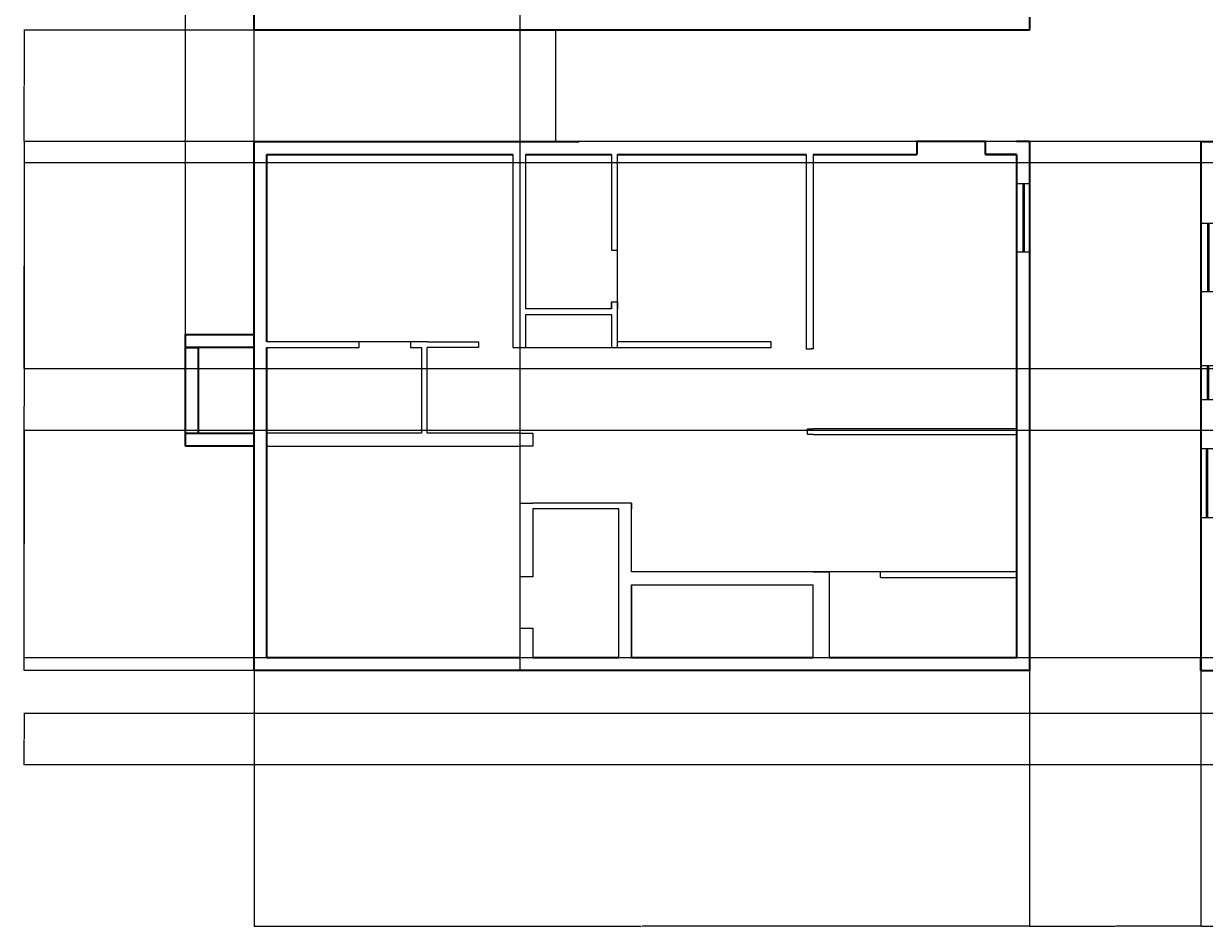
# Model space of a CAD drawing. Units: inches. Extents: x 2029 to 8798, y 1998 to 6373.
# Tile 1 of 11: x 2029 to 2855, y 4031 to 4662. Entities that reach past the tile are written whole.
import ezdxf

# ---------------------------------------------------------------- set-up
doc = ezdxf.new("R2010")
doc.units = ezdxf.units.IN
for name, color, linetype, lineweight in [('A-ANNO-DIMS', 2, 'Continuous', 18), ('A-GLAZ', 4, 'Continuous', 18), ('A-WALL-CIRC', 7, 'Continuous', 25), ('A-WALL-EXTR', 7, 'Continuous', 35), ('A-WALL-INTR', 7, 'Continuous', 25)]:
    doc.layers.add(name, color=color, linetype=linetype, lineweight=lineweight)
doc.styles.get("Standard").update_dxf_attribs({"font": 'arial.ttf'})
doc.dimstyles.get("Standard").update_dxf_attribs({"dimtxt": 0.18, "dimasz": 0.18, "dimexe": 0.18, "dimexo": 0.0625, "dimgap": 0.09, "dimtad": 0, "dimtih": 1, "dimtoh": 1, "dimdec": 4, "dimzin": 0, "dimdsep": 46, "dimtxsty": 'Standard', "dimcen": 0.09, "dimadec": 0, "dimazin": 0, "dimtfac": 1, "dimtdec": 4, "dimtofl": 0, "dimtmove": 0, "dimatfit": 3, "dimfxl": 1, "dimtolj": 1, "dimtzin": 0, "dimarcsym": 0})

# ---------------------------------------------------------------- blocks, each defined once
blk = doc.blocks.new('WIN-48')
for p, q in [((0, 48), (9, 48)), ((4.5, 48), (4.5, 0)), ((5.5, 48), (5.5, 0)), ((9, 0), (0, 0))]:
    blk.add_line(p, q)
blk = doc.blocks.new('WIN-24')
for p, q in [((0, 0), (0, 9)), ((24, 9), (24, 0)), ((0, 4.5), (24, 4.5)), ((0, 3.5), (24, 3.5))]:
    blk.add_line(p, q)
blk = doc.blocks.new('WALL-BAY-78X48')
for p, q in [((0, 69), (0, 78)), ((0, 78), (48, 78)), ((48, 69), (0, 69)), ((0, 9), (0, 69)), ((0, 69), (9, 69)), ((9, 69), (9, 9)), ((0, 0), (0, 9)), ((0, 9), (48, 9)), ((48, 0), (0, 0))]:
    blk.add_line(p, q)
blk = doc.blocks.new('*D37')
at = {"layer": 'A-ANNO-DIMS', "color": 0, "lineweight": -2, "transparency": 16777216}
for p, q in [((2190.54, 4209.93), (2190.54, 4031.06)), ((2732.54, 4209.93), (2732.54, 4031.06)), ((2190.72, 4031.24), (2461.25, 4031.24)), ((2732.36, 4031.24), (2461.83, 4031.24))]:
    blk.add_line(p, q, dxfattribs=at)
at = {"layer": 'A-ANNO-DIMS', "color": 0, "transparency": 16777216}
for points in [[(2190.72, 4031.27), (2190.72, 4031.21), (2190.54, 4031.24)], [(2732.36, 4031.27), (2732.36, 4031.21), (2732.54, 4031.24)]]:
    blk.add_solid(points, dxfattribs=at)
at = {"layer": 'Defpoints', "color": 0, "transparency": 16777216}
for p in [(2190.54, 4209.99), (2732.54, 4209.99), (2732.54, 4031.24)]:
    blk.add_point(p, dxfattribs=at)
at = {"layer": 'A-ANNO-DIMS', "color": 0, "transparency": 16777216, "insert": (2461.54, 4031.24), "char_height": 0.18, "attachment_point": 5}
blk.add_mtext('\\A1;542', dxfattribs=at)
blk = doc.blocks.new('*D38')
at = {"layer": 'A-ANNO-DIMS', "color": 0, "lineweight": -2, "transparency": 16777216}
for p, q in [((2732.54, 4209.93), (2732.54, 4031.06)), ((2852.54, 4209.93), (2852.54, 4031.06)), ((2732.72, 4031.24), (2792.26, 4031.24)), ((2852.36, 4031.24), (2792.82, 4031.24))]:
    blk.add_line(p, q, dxfattribs=at)
at = {"layer": 'A-ANNO-DIMS', "color": 0, "transparency": 16777216}
for points in [[(2732.72, 4031.27), (2732.72, 4031.21), (2732.54, 4031.24)], [(2852.36, 4031.27), (2852.36, 4031.21), (2852.54, 4031.24)]]:
    blk.add_solid(points, dxfattribs=at)
at = {"layer": 'Defpoints', "color": 0, "transparency": 16777216}
for p in [(2732.54, 4209.99), (2852.54, 4209.99), (2852.54, 4031.24)]:
    blk.add_point(p, dxfattribs=at)
at = {"layer": 'A-ANNO-DIMS', "color": 0, "transparency": 16777216, "insert": (2792.54, 4031.24), "char_height": 0.18, "attachment_point": 5}
blk.add_mtext('\\A1;120', dxfattribs=at)
blk = doc.blocks.new('*D39')
at = {"layer": 'A-ANNO-DIMS', "color": 0, "lineweight": -2, "transparency": 16777216}
for p, q in [((2852.54, 4209.93), (2852.54, 4031.06)), ((3252.54, 4209.93), (3252.54, 4031.06)), ((2852.72, 4031.24), (3052.25, 4031.24)), ((3252.36, 4031.24), (3052.83, 4031.24))]:
    blk.add_line(p, q, dxfattribs=at)
at = {"layer": 'A-ANNO-DIMS', "color": 0, "transparency": 16777216}
for points in [[(2852.72, 4031.27), (2852.72, 4031.21), (2852.54, 4031.24)], [(3252.36, 4031.27), (3252.36, 4031.21), (3252.54, 4031.24)]]:
    blk.add_solid(points, dxfattribs=at)
at = {"layer": 'Defpoints', "color": 0, "transparency": 16777216}
for p in [(2852.54, 4209.99), (3252.54, 4209.99), (3252.54, 4031.24)]:
    blk.add_point(p, dxfattribs=at)
at = {"layer": 'A-ANNO-DIMS', "color": 0, "transparency": 16777216, "insert": (3052.54, 4031.24), "char_height": 0.18, "attachment_point": 5}
blk.add_mtext('\\A1;400', dxfattribs=at)
blk = doc.blocks.new('*D43')
at = {"layer": 'A-ANNO-DIMS', "color": 0, "lineweight": -2, "transparency": 16777216}
for p, q in [((2190.48, 4579.99), (2029.61, 4579.99)), ((2029.79, 4579.81), (2029.79, 4395.17)), ((2029.79, 4210.17), (2029.79, 4394.81)), ((2190.48, 4209.99), (2029.61, 4209.99))]:
    blk.add_line(p, q, dxfattribs=at)
at = {"layer": 'A-ANNO-DIMS', "color": 0, "transparency": 16777216}
for points in [[(2029.76, 4579.81), (2029.82, 4579.81), (2029.79, 4579.99)], [(2029.76, 4210.17), (2029.82, 4210.17), (2029.79, 4209.99)]]:
    blk.add_solid(points, dxfattribs=at)
at = {"layer": 'Defpoints', "color": 0, "transparency": 16777216}
for p in [(2029.79, 4579.99), (2190.54, 4579.99), (2190.54, 4209.99)]:
    blk.add_point(p, dxfattribs=at)
at = {"layer": 'A-ANNO-DIMS', "color": 0, "transparency": 16777216, "insert": (2029.79, 4394.99), "char_height": 0.18, "attachment_point": 5}
blk.add_mtext('\\A1;370', dxfattribs=at)
blk = doc.blocks.new('*D44')
at = {"layer": 'A-ANNO-DIMS', "color": 0, "lineweight": -2, "transparency": 16777216}
for p, q in [((2190.48, 4657.96), (2029.61, 4657.96)), ((2029.79, 4657.78), (2029.79, 4619.16)), ((2029.79, 4580.17), (2029.79, 4618.79)), ((2190.48, 4579.99), (2029.61, 4579.99))]:
    blk.add_line(p, q, dxfattribs=at)
at = {"layer": 'A-ANNO-DIMS', "color": 0, "transparency": 16777216}
for points in [[(2029.76, 4657.78), (2029.82, 4657.78), (2029.79, 4657.96)], [(2029.76, 4580.17), (2029.82, 4580.17), (2029.79, 4579.99)]]:
    blk.add_solid(points, dxfattribs=at)
at = {"layer": 'Defpoints', "color": 0, "transparency": 16777216}
for p in [(2029.79, 4657.96), (2190.54, 4657.96), (2190.54, 4579.99)]:
    blk.add_point(p, dxfattribs=at)
at = {"layer": 'A-ANNO-DIMS', "color": 0, "transparency": 16777216, "insert": (2029.79, 4618.97), "char_height": 0.18, "attachment_point": 5}
blk.add_mtext('\\A1;77.97', dxfattribs=at)
blk = doc.blocks.new('*D49')
at = {"layer": 'A-ANNO-DIMS', "color": 0, "lineweight": -2, "transparency": 16777216}
for p, q in [((2190.54, 4210.05), (2190.54, 6372.54)), ((2190.72, 6372.36), (2283.26, 6372.36)), ((2376.36, 6372.36), (2283.82, 6372.36)), ((2376.54, 4210.05), (2376.54, 6372.54))]:
    blk.add_line(p, q, dxfattribs=at)
at = {"layer": 'A-ANNO-DIMS', "color": 0, "transparency": 16777216}
for points in [[(2190.72, 6372.39), (2190.72, 6372.33), (2190.54, 6372.36)], [(2376.36, 6372.39), (2376.36, 6372.33), (2376.54, 6372.36)]]:
    blk.add_solid(points, dxfattribs=at)
at = {"layer": 'Defpoints', "color": 0, "transparency": 16777216}
for p in [(2376.54, 6372.36), (2190.54, 4209.99), (2376.54, 4209.99)]:
    blk.add_point(p, dxfattribs=at)
at = {"layer": 'A-ANNO-DIMS', "color": 0, "transparency": 16777216, "insert": (2283.54, 6372.36), "char_height": 0.18, "attachment_point": 5}
blk.add_mtext('\\A1;186', dxfattribs=at)
blk = doc.blocks.new('*D50')
at = {"layer": 'A-ANNO-DIMS', "color": 0, "lineweight": -2, "transparency": 16777216}
for p, q in [((2852.54, 4579.93), (2852.54, 4031.06)), ((3006.54, 4579.93), (3006.54, 4031.06)), ((2852.72, 4031.24), (2929.26, 4031.24)), ((3006.36, 4031.24), (2929.82, 4031.24))]:
    blk.add_line(p, q, dxfattribs=at)
at = {"layer": 'A-ANNO-DIMS', "color": 0, "transparency": 16777216}
for points in [[(2852.72, 4031.27), (2852.72, 4031.21), (2852.54, 4031.24)], [(3006.36, 4031.27), (3006.36, 4031.21), (3006.54, 4031.24)]]:
    blk.add_solid(points, dxfattribs=at)
at = {"layer": 'Defpoints', "color": 0, "transparency": 16777216}
for p in [(2852.54, 4579.99), (3006.54, 4579.99), (3006.54, 4031.24)]:
    blk.add_point(p, dxfattribs=at)
at = {"layer": 'A-ANNO-DIMS', "color": 0, "transparency": 16777216, "insert": (2929.54, 4031.24), "char_height": 0.18, "attachment_point": 5}
blk.add_mtext('\\A1;154', dxfattribs=at)
blk = doc.blocks.new('*D53')
at = {"layer": 'A-ANNO-DIMS', "color": 0, "lineweight": -2, "transparency": 16777216}
for p, q in [((2861.48, 4377.99), (2029.61, 4377.99)), ((2029.79, 4377.81), (2029.79, 4298.67)), ((2029.79, 4219.17), (2029.79, 4298.31)), ((2861.48, 4218.99), (2029.61, 4218.99))]:
    blk.add_line(p, q, dxfattribs=at)
at = {"layer": 'A-ANNO-DIMS', "color": 0, "transparency": 16777216}
for points in [[(2029.76, 4377.81), (2029.82, 4377.81), (2029.79, 4377.99)], [(2029.76, 4219.17), (2029.82, 4219.17), (2029.79, 4218.99)]]:
    blk.add_solid(points, dxfattribs=at)
at = {"layer": 'Defpoints', "color": 0, "transparency": 16777216}
for p in [(2861.54, 4377.99), (2029.79, 4218.99), (2861.54, 4218.99)]:
    blk.add_point(p, dxfattribs=at)
at = {"layer": 'A-ANNO-DIMS', "color": 0, "transparency": 16777216, "insert": (2029.79, 4298.49), "char_height": 0.18, "attachment_point": 5}
blk.add_mtext('\\A1;159', dxfattribs=at)
blk = doc.blocks.new('*D86')
at = {"layer": 'A-ANNO-DIMS', "color": 0, "lineweight": -2, "transparency": 16777216}
for p, q in [((4373.7, 4564.99), (2029.61, 4564.99)), ((2029.79, 4564.81), (2029.79, 4493.17)), ((2029.79, 4421.17), (2029.79, 4492.81)), ((4373.7, 4420.99), (2029.61, 4420.99))]:
    blk.add_line(p, q, dxfattribs=at)
at = {"layer": 'A-ANNO-DIMS', "color": 0, "transparency": 16777216}
for points in [[(2029.76, 4564.81), (2029.82, 4564.81), (2029.79, 4564.99)], [(2029.76, 4421.17), (2029.82, 4421.17), (2029.79, 4420.99)]]:
    blk.add_solid(points, dxfattribs=at)
at = {"layer": 'Defpoints', "color": 0, "transparency": 16777216}
for p in [(4373.77, 4564.99), (2029.79, 4420.99), (4373.77, 4420.99)]:
    blk.add_point(p, dxfattribs=at)
at = {"layer": 'A-ANNO-DIMS', "color": 0, "transparency": 16777216, "insert": (2029.79, 4492.99), "char_height": 0.18, "attachment_point": 5}
blk.add_mtext('\\A1;144', dxfattribs=at)
blk = doc.blocks.new('*D88')
at = {"layer": 'A-ANNO-DIMS', "color": 0, "lineweight": -2, "transparency": 16777216}
for p, q in [((2142.54, 4445.05), (2142.54, 6372.54)), ((2142.72, 6372.36), (3266.19, 6372.36)), ((4390.59, 6372.36), (3267.12, 6372.36)), ((4390.77, 4574.05), (4390.77, 6372.54))]:
    blk.add_line(p, q, dxfattribs=at)
at = {"layer": 'A-ANNO-DIMS', "color": 0, "transparency": 16777216}
for points in [[(2142.72, 6372.39), (2142.72, 6372.33), (2142.54, 6372.36)], [(4390.59, 6372.39), (4390.59, 6372.33), (4390.77, 6372.36)]]:
    blk.add_solid(points, dxfattribs=at)
at = {"layer": 'Defpoints', "color": 0, "transparency": 16777216}
for p in [(4390.77, 6372.36), (4390.77, 4573.99), (2142.54, 4444.99)]:
    blk.add_point(p, dxfattribs=at)
at = {"layer": 'A-ANNO-DIMS', "color": 0, "transparency": 16777216, "insert": (3266.65, 6372.36), "char_height": 0.18, "attachment_point": 5}
blk.add_mtext('\\A1;2248.2', dxfattribs=at)
blk = doc.blocks.new('*D117')
at = {"layer": 'A-ANNO-DIMS', "color": 0, "lineweight": -2, "transparency": 16777216}
for p, q in [((4105.7, 4179.99), (2029.61, 4179.99)), ((2029.79, 4179.81), (2029.79, 4162.17)), ((2029.79, 4144.17), (2029.79, 4161.81)), ((4105.7, 4143.99), (2029.61, 4143.99))]:
    blk.add_line(p, q, dxfattribs=at)
at = {"layer": 'A-ANNO-DIMS', "color": 0, "transparency": 16777216}
for points in [[(2029.76, 4179.81), (2029.82, 4179.81), (2029.79, 4179.99)], [(2029.76, 4144.17), (2029.82, 4144.17), (2029.79, 4143.99)]]:
    blk.add_solid(points, dxfattribs=at)
at = {"layer": 'Defpoints', "color": 0, "transparency": 16777216}
for p in [(2029.79, 4179.99), (4105.77, 4179.99), (4105.77, 4143.99)]:
    blk.add_point(p, dxfattribs=at)
at = {"layer": 'A-ANNO-DIMS', "color": 0, "transparency": 16777216, "insert": (2029.79, 4161.99), "char_height": 0.18, "attachment_point": 5}
blk.add_mtext('\\A1;36', dxfattribs=at)

msp = doc.modelspace()

# ---------------------------------------------------------------- linework, layer by layer
at = {"layer": 'A-GLAZ'}
for p, q in [((2852.5398, 4474.9886), (2852.5398, 4522.9886)), ((2852.5398, 4399.2558), (2852.5398, 4423.2558)), ((2852.5398, 4365.0621), (2852.5398, 4317.0621))]:
    msp.add_line(p, q, dxfattribs=at)
at = {"layer": 'A-WALL-CIRC'}
for p, q in [((2401.3042, 4657.9886), (2401.3042, 4579.9886)), ((3006.5398, 4579.9886), (2417.7365, 4579.9886)), ((2852.5398, 4579.9886), (2712.1381, 4579.9886)), ((2852.5398, 4579.9886), (2732.5398, 4579.9886))]:
    msp.add_line(p, q, dxfattribs=at)
at = {"layer": 'A-WALL-EXTR'}
for p, q in [((2190.5398, 4657.9585), (2190.5398, 5027.9585)), ((2732.5398, 4666.9886), (2732.5398, 4657.9585)), ((2199.5398, 4657.9585), (2190.5398, 4657.9585)), ((2367.5398, 4657.9585), (2199.5398, 4657.9585)), ((2376.5398, 4657.9585), (2367.5398, 4657.9585)), ((2436.5398, 4657.9585), (2376.5398, 4657.9585)), ((2732.5398, 4657.9886), (2402.4452, 4657.9886)), ((2445.5398, 4657.9585), (2436.5398, 4657.9585)), ((2572.5398, 4657.9585), (2445.5398, 4657.9585)), ((2581.5398, 4657.9585), (2572.5398, 4657.9585)), ((2723.5398, 4657.9585), (2581.5398, 4657.9585)), ((2723.5398, 4657.9585), (2723.5398, 4657.9886)), ((2732.5398, 4657.9585), (2723.5398, 4657.9585)), ((2732.5398, 4657.9886), (2732.5398, 4657.9585)), ((2190.5398, 4209.9886), (2190.5398, 4579.9886)), ((2190.5398, 4579.9886), (2401.3042, 4579.9886)), ((2401.3042, 4579.9886), (2417.7365, 4579.9886)), ((2701.9545, 4579.9886), (2653.9545, 4579.9886)), ((2653.9545, 4579.9886), (2653.9545, 4570.9886)), ((2701.9545, 4570.9886), (2701.9545, 4579.9886)), ((2732.5398, 4579.9886), (2723.5398, 4579.9886)), ((2732.5398, 4579.9886), (2723.5398, 4579.9886)), ((2732.5398, 4579.9886), (2732.5398, 4209.9886)), ((2852.5398, 4579.9886), (2852.5398, 4570.9886)), ((2852.5398, 4579.9886), (2861.5398, 4579.9886)), ((2199.5398, 4570.9886), (2371.5398, 4570.9886)), ((2199.5398, 4570.9886), (2371.5398, 4570.9886)), ((2199.5398, 4439.9886), (2199.5398, 4570.9886)), ((2380.5398, 4570.9886), (2440.5398, 4570.9886)), ((2380.5398, 4570.9886), (2440.5398, 4570.9886)), ((2444.5398, 4570.9886), (2576.5398, 4570.9886)), ((2444.5398, 4570.9886), (2576.5398, 4570.9886)), ((2581.5398, 4570.9886), (2653.9545, 4570.9886)), ((2723.5398, 4570.9886), (2701.9545, 4570.9886)), ((2701.9545, 4570.9886), (2723.5398, 4570.9886)), ((2723.5398, 4570.9886), (2723.5398, 4550.5639)), ((2852.5398, 4570.9886), (2852.5398, 4450.9886)), ((2723.5398, 4550.5639), (2723.5398, 4500.7607)), ((2723.5398, 4502.5639), (2723.5398, 4218.9886)), ((2723.5398, 4502.5639), (2723.5398, 4378.9886)), ((2852.5398, 4450.9886), (2852.5398, 4441.9886)), ((2852.5398, 4441.9886), (2852.5398, 4381.9886)), ((2199.5398, 4218.9886), (2199.5398, 4435.9886)), ((2199.5398, 4375.9886), (2199.5398, 4435.9886)), ((2723.5398, 4374.9886), (2723.5398, 4278.9886)), ((2852.5398, 4381.9886), (2852.5398, 4377.9886)), ((2852.5398, 4377.9886), (2852.5398, 4218.9886)), ((2199.5398, 4218.9886), (2199.5398, 4366.9886)), ((2376.5398, 4218.9886), (2199.5398, 4218.9886)), ((2445.5398, 4218.9886), (2385.5398, 4218.9886)), ((2581.5398, 4218.9886), (2454.5398, 4218.9886)), ((2723.5398, 4218.9886), (2592.544, 4218.9886)), ((2723.5398, 4218.9886), (2592.544, 4218.9886)), ((2852.5398, 4218.9886), (2852.5398, 4209.9886)), ((2852.5398, 4209.9886), (2852.5398, 4218.9886)), ((2199.5398, 4209.9886), (2190.5398, 4209.9886)), ((2367.5398, 4209.9886), (2199.5398, 4209.9886)), ((2376.5398, 4209.9886), (2367.5398, 4209.9886)), ((2436.5398, 4209.9886), (2376.5398, 4209.9886)), ((2445.5398, 4209.9886), (2436.5398, 4209.9886)), ((2572.5398, 4209.9886), (2445.5398, 4209.9886)), ((2581.5398, 4209.9886), (2572.5398, 4209.9886)), ((2723.5398, 4209.9886), (2581.5398, 4209.9886)), ((2732.5398, 4209.9886), (2723.5398, 4209.9886)), ((2852.5398, 4209.9886), (2861.5398, 4209.9886))]:
    msp.add_line(p, q, dxfattribs=at)
at = {"layer": 'A-WALL-INTR'}
for p, q in [((2371.5398, 4570.9886), (2371.5398, 4435.9886)), ((2380.5398, 4462.9886), (2380.5398, 4570.9886)), ((2440.5398, 4570.9886), (2440.5398, 4503.9871)), ((2444.5398, 4462.9886), (2444.5398, 4570.9886)), ((2576.5398, 4570.9886), (2576.5398, 4434.9886)), ((2581.5398, 4570.9886), (2581.5398, 4434.9886)), ((2440.5398, 4503.9871), (2444.5398, 4503.9871)), ((2440.5398, 4462.9886), (2440.5398, 4467.9871)), ((2440.5398, 4467.9871), (2444.5398, 4467.9871)), ((2440.5398, 4467.9871), (2440.5398, 4462.9886)), ((2444.5398, 4467.9871), (2444.5398, 4462.9886)), ((2440.5398, 4462.9886), (2380.5398, 4462.9886)), ((2380.5398, 4435.9886), (2380.5398, 4458.9886)), ((2380.5398, 4458.9886), (2440.4529, 4458.9886)), ((2440.4529, 4458.9886), (2440.4529, 4435.9886)), ((2444.5398, 4458.9886), (2444.5398, 4462.9886)), ((2444.5398, 4435.9886), (2444.5398, 4458.9886)), ((2307.5398, 4439.9886), (2199.5398, 4439.9886)), ((2199.5398, 4435.9886), (2264.03, 4435.9886)), ((2264.03, 4435.9886), (2264.03, 4439.9886)), ((2307.5398, 4439.9886), (2300.03, 4439.9886)), ((2300.03, 4439.9886), (2300.03, 4435.9886)), ((2300.03, 4435.9886), (2307.5398, 4435.9886)), ((2311.5398, 4439.9886), (2307.5398, 4439.9886)), ((2307.5398, 4435.9886), (2307.5398, 4375.9886)), ((2311.5398, 4439.9886), (2347.5398, 4439.9886)), ((2311.5398, 4375.9886), (2311.5398, 4435.9886)), ((2347.5398, 4435.9886), (2311.5398, 4435.9886)), ((2347.5398, 4439.9886), (2347.5398, 4435.9886)), ((2371.5398, 4435.9886), (2380.5398, 4435.9886)), ((2380.5398, 4435.9886), (2444.5398, 4435.9886)), ((2440.4529, 4435.9886), (2444.5398, 4435.9886)), ((2552.1143, 4439.9886), (2444.5398, 4439.9886)), ((2444.5398, 4435.9886), (2552.1143, 4435.9886)), ((2552.1143, 4435.9886), (2552.1143, 4439.9886)), ((2576.5398, 4434.9886), (2580.5398, 4434.9886)), ((2581.5398, 4434.9886), (2579.9704, 4434.9886)), ((2307.5398, 4375.9886), (2199.5398, 4375.9886)), ((2376.5398, 4375.9886), (2311.5398, 4375.9886)), ((2376.5398, 4375.9886), (2385.5398, 4375.9886)), ((2385.5398, 4375.9886), (2385.5398, 4366.9886)), ((2577.5398, 4374.9886), (2577.5398, 4378.9886)), ((2577.5398, 4378.9886), (2581.5398, 4378.9886)), ((2581.5398, 4374.9886), (2577.5398, 4374.9886)), ((2723.5398, 4378.9886), (2581.5398, 4378.9886)), ((2581.5398, 4374.9886), (2723.5398, 4374.9886)), ((2199.5398, 4366.9886), (2376.5398, 4366.9886)), ((2385.5398, 4366.9886), (2376.5398, 4366.9886)), ((2376.5398, 4218.9886), (2376.5398, 4326.9886)), ((2376.5398, 4326.9886), (2385.5398, 4326.9886)), ((2445.5398, 4326.9886), (2385.5398, 4326.9886)), ((2454.5398, 4326.9886), (2445.5398, 4326.9886)), ((2454.5398, 4278.9886), (2454.5398, 4326.9886)), ((2454.5398, 4326.9886), (2454.5398, 4322.9886)), ((2385.5398, 4322.9886), (2385.5398, 4275.6599)), ((2445.5398, 4322.9886), (2385.5398, 4322.9886)), ((2445.5398, 4218.9886), (2445.5398, 4322.9886)), ((2445.5398, 4218.9886), (2445.5398, 4278.9886)), ((2454.5398, 4278.9886), (2454.5398, 4279.9886)), ((2581.5398, 4278.9886), (2454.5398, 4278.9886)), ((2723.5398, 4278.9886), (2581.5398, 4278.9886)), ((2581.5398, 4278.9886), (2592.544, 4278.9886)), ((2592.544, 4278.9886), (2592.544, 4274.9886)), ((2628.544, 4274.9886), (2628.544, 4278.9886)), ((2385.5398, 4275.6599), (2376.5398, 4275.6599)), ((2454.5398, 4269.9886), (2454.5398, 4218.9886)), ((2454.5398, 4218.9886), (2454.5398, 4269.9886)), ((2454.5398, 4269.9886), (2581.5398, 4269.9886)), ((2581.5398, 4218.9886), (2581.5398, 4269.9886)), ((2592.544, 4274.9886), (2592.544, 4218.9886)), ((2628.544, 4274.9886), (2723.5398, 4274.9886)), ((2376.5398, 4218.9886), (2376.5398, 4239.6599)), ((2376.5398, 4239.6599), (2385.5398, 4239.6599)), ((2385.5398, 4239.6599), (2385.5398, 4218.9886))]:
    msp.add_line(p, q, dxfattribs=at)

# ---------------------------------------------------------------- block references
at = {"layer": 'A-GLAZ'}
for p in [(2723.5398, 4502.5639), (2852.5398, 4474.9886)]:
    msp.add_blockref('WIN-48', p, dxfattribs=at)
at = {"layer": 'A-GLAZ', "rotation": 90}
msp.add_blockref('WIN-24', (2861.5398, 4399.2558), dxfattribs=at)
at = {"layer": 'A-GLAZ', "extrusion": (0, 0, -1), "zscale": -1}
msp.add_blockref('WIN-48', (-2861.5398, 4317.0621), dxfattribs=at)
at = {"layer": 'A-WALL-EXTR'}
msp.add_blockref('WALL-BAY-78X48', (2142.5398, 4366.9886), dxfattribs=at)

# ---------------------------------------------------------------- dimensions: what is measured, and where the dimension line sits
at = {"layer": 'A-ANNO-DIMS'}
for base, p1, p2, override, picture, middle in [((4390.7657, 6372.3623), (2142.5398, 4444.9886), (4390.7657, 4573.9886), {"dimdec": 1, "dimlfac": 1, "dimrnd": 0, "dimzin": 0, "dimdsep": 46, "dimlunit": 2}, '*D88', (3266.6528, 6372.3623)), ((2376.5398, 6372.3623), (2190.5398, 4209.9886), (2376.5398, 4209.9886), {"dimdec": 0, "dimlfac": 1, "dimrnd": 0, "dimzin": 0, "dimdsep": 46, "dimlunit": 2}, '*D49', (2283.5398, 6372.3623)), ((3006.5398, 4031.2386), (2852.5398, 4579.9886), (3006.5398, 4579.9886), {"dimdec": 0, "dimlfac": 1, "dimrnd": 0, "dimzin": 0, "dimdsep": 46, "dimlunit": 2}, '*D50', (2929.5398, 4031.2386)), ((2732.5398, 4031.2386), (2190.5398, 4209.9886), (2732.5398, 4209.9886), {"dimdec": 0, "dimlfac": 1, "dimrnd": 0, "dimzin": 0, "dimdsep": 46, "dimlunit": 2}, '*D37', (2461.5398, 4031.2386)), ((2852.5398, 4031.2386), (2732.5398, 4209.9886), (2852.5398, 4209.9886), {"dimdec": 0, "dimlfac": 1, "dimrnd": 0, "dimzin": 0, "dimdsep": 46, "dimlunit": 2}, '*D38', (2792.5398, 4031.2386)), ((3252.5398, 4031.2386), (2852.5398, 4209.9886), (3252.5398, 4209.9886), {"dimdec": 0, "dimlfac": 1, "dimrnd": 0, "dimzin": 0, "dimdsep": 46, "dimlunit": 2}, '*D39', (3052.5398, 4031.2386))]:
    dim = msp.add_linear_dim(base=base, p1=p1, p2=p2, dimstyle='Standard', override=override, dxfattribs=at)
    dim.commit()
    dim.dimension.update_dxf_attribs({"geometry": picture, "text_midpoint": middle})
for base, p1, p2, override, picture, middle in [((2029.7898, 4657.9585), (2190.5398, 4579.9886), (2190.5398, 4657.9585), {"dimdec": 2, "dimlfac": 1, "dimrnd": 0, "dimzin": 0, "dimdsep": 46, "dimlunit": 2}, '*D44', (2029.7898, 4618.9735)), ((2029.7898, 4579.9886), (2190.5398, 4209.9886), (2190.5398, 4579.9886), {"dimdec": 0, "dimlfac": 1, "dimrnd": 0, "dimzin": 0, "dimdsep": 46, "dimlunit": 2}, '*D43', (2029.7898, 4394.9886)), ((2029.7898, 4420.9886), (4373.7657, 4564.9886), (4373.7657, 4420.9886), {"dimdec": 0, "dimlfac": 1, "dimrnd": 0, "dimzin": 0, "dimdsep": 46, "dimlunit": 2}, '*D86', (2029.7898, 4492.9886)), ((2029.7898, 4218.9886), (2861.5398, 4377.9886), (2861.5398, 4218.9886), {"dimdec": 0, "dimlfac": 1, "dimrnd": 0, "dimzin": 0, "dimdsep": 46, "dimlunit": 2}, '*D53', (2029.7898, 4298.4886)), ((2029.7898, 4179.9886), (4105.7657, 4143.9886), (4105.7657, 4179.9886), {"dimdec": 0, "dimlfac": 1, "dimrnd": 0, "dimzin": 0, "dimdsep": 46, "dimlunit": 2}, '*D117', (2029.7898, 4161.9886))]:
    dim = msp.add_linear_dim(base=base, p1=p1, p2=p2, angle=90, dimstyle='Standard', override=override, dxfattribs=at)
    dim.commit()
    dim.dimension.update_dxf_attribs({"geometry": picture, "text_midpoint": middle})

doc.saveas('drawing.dxf')
